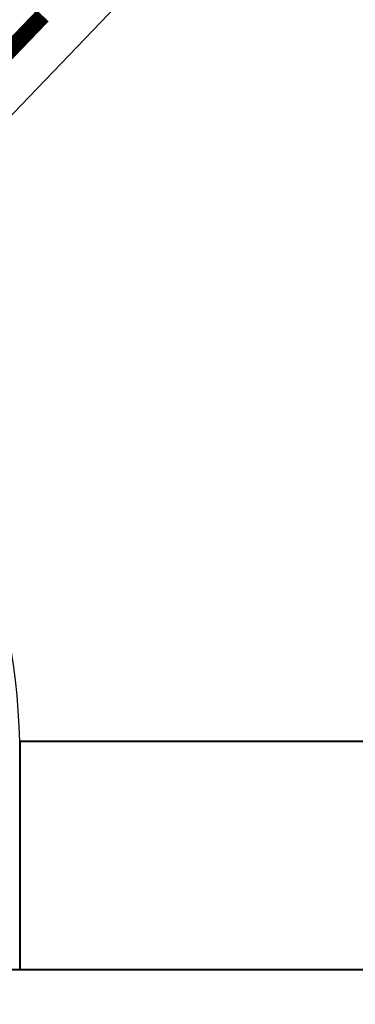
# Model space of a CAD drawing. Units: inches. Extents: x 459864 to 460310, y 324185 to 324787.
# Tile 64 of 112: x 460088 to 460101, y 324282 to 324321. Entities that reach past the tile are written whole.
import ezdxf

# ---------------------------------------------------------------- set-up
doc = ezdxf.new("R2010")
doc.units = ezdxf.units.IN
for name, color, linetype, lineweight in [('A-ANNO-DIMS', 2, 'Continuous', 18), ('A-DOOR', 3, 'Continuous', 25), ('A-WALL', 7, 'Continuous', 40), ('L-SITE-PATT', 252, 'Continuous', 13)]:
    doc.layers.add(name, color=color, linetype=linetype, lineweight=lineweight)
doc.styles.get("Standard").update_dxf_attribs({"font": 'arial.ttf'})
doc.dimstyles.new('ISO-25', dxfattribs={"dimtxt": 6, "dimasz": 2.5, "dimexe": 1.25, "dimexo": 0.625, "dimtad": 1, "dimdec": 1, "dimlunit": 3, "dimtxsty": 'Standard', "dimcen": 2.5, "dimadec": 0, "dimazin": 0, "dimtfac": 1, "dimtdec": 1, "dimtmove": 0, "dimatfit": 3, "dimfxl": 1, "dimarcsym": 0})

# ---------------------------------------------------------------- blocks, each defined once
blk = doc.blocks.new('*D73')
at = {"layer": 'A-ANNO-DIMS', "color": 0, "lineweight": -2, "transparency": 16777216}
for p, q in [((460109.617, 324339.904), (460082.316, 324311.465)), ((460063.615, 324291.983), (460080.585, 324309.661))]:
    blk.add_line(p, q, dxfattribs=at)
at = {"layer": 'A-ANNO-DIMS', "color": 0, "transparency": 16777216}
blk.add_solid([(460082.016, 324311.753), (460082.617, 324311.176), (460080.585, 324309.661)], dxfattribs=at)
at = {"layer": 'Defpoints', "color": 0, "transparency": 16777216}
for p in [(460080.585, 324309.661), (460063.615, 324291.983)]:
    blk.add_point(p, dxfattribs=at)
at = {"layer": 'A-ANNO-DIMS', "color": 0, "transparency": 16777216, "insert": (460094.144, 324329.167), "char_height": 6, "attachment_point": 5, "rotation": 46.1701}
blk.add_mtext('R2\'-0 1/2"', dxfattribs=at)

msp = doc.modelspace()

# ---------------------------------------------------------------- hatches: boundary and pattern name
at = {"layer": 'L-SITE-PATT'}
h = msp.add_hatch(dxfattribs=at)
h.set_pattern_fill('DOTS', color=256)
h.paths.add_polyline_path([(460269.804, 324283.483), (460247.115, 324283.483), (460121.929, 324283.483), (460121.929, 324252.473), (460117.429, 324252.473), (460110.124, 324252.473), (460110.124, 324243.287), (460080.83, 324243.287), (460080.83, 324252.473), (460061.115, 324252.473), (460061.115, 324251.882), (460077.909, 324251.882), (460077.909, 324199.483), (460080.83, 324199.483), (460080.83, 324207.553), (460110.124, 324207.553), (460110.124, 324199.483), (460110.813, 324199.483), (460262.115, 324199.483), (460269.804, 324199.483)], flags=17)
edge = h.paths.add_edge_path(flags=0)
edge.add_ellipse((460222.59, 324263.813), major_axis=(-8.485, 8.485), ratio=1, start_angle=405, end_angle=495, ccw=False)
edge.add_line((460214.821, 324254.66), (460214.832, 324254.666))
edge.add_ellipse((460222.59, 324263.813), major_axis=(-8.485, 8.485), ratio=1, start_angle=405, end_angle=495, ccw=False)
edge.add_line((460210.759, 324261.781), (460210.768, 324261.787))
edge.add_ellipse((460222.59, 324263.813), major_axis=(-8.485, 8.485), ratio=1, start_angle=405, end_angle=495, ccw=False)
edge.add_ellipse((460222.59, 324263.813), major_axis=(-8.485, 8.485), ratio=1, start_angle=392.754, end_angle=405, ccw=False)
edge.add_ellipse((460222.59, 324263.813), major_axis=(-8.485, 8.485), ratio=1, start_angle=380.9347, end_angle=392.754, ccw=False)
edge.add_line((460211.337, 324267.985), (460211.34, 324267.985))
edge.add_ellipse((460222.59, 324263.813), major_axis=(-8.485, 8.485), ratio=1, start_angle=380.9347, end_angle=392.754, ccw=False)
edge.add_ellipse((460222.59, 324263.813), major_axis=(-8.485, 8.485), ratio=1, start_angle=347.9015, end_angle=380.9347, ccw=False)
edge.add_ellipse((460222.59, 324263.813), major_axis=(-8.485, 8.485), ratio=1, start_angle=327.0619, end_angle=347.9015, ccw=False)
edge.add_ellipse((460222.59, 324263.813), major_axis=(-8.485, 8.485), ratio=1, start_angle=278.3246, end_angle=327.0619, ccw=False)
edge.add_line((460225.158, 324275.536), (460225.158, 324275.535))
edge.add_ellipse((460222.59, 324263.813), major_axis=(-8.485, 8.485), ratio=1, start_angle=278.3246, end_angle=327.0619, ccw=False)
edge.add_ellipse((460222.59, 324263.813), major_axis=(-8.485, 8.485), ratio=1, start_angle=260.6436, end_angle=278.3246, ccw=False)
edge.add_ellipse((460222.59, 324263.813), major_axis=(-8.485, 8.485), ratio=1, start_angle=225, end_angle=260.6436, ccw=False)
edge.add_line((460234.509, 324265.243), (460234.501, 324265.239))
edge.add_ellipse((460222.59, 324263.813), major_axis=(-8.485, 8.485), ratio=1, start_angle=225, end_angle=260.6436, ccw=False)
edge.add_ellipse((460222.59, 324263.813), major_axis=(-8.485, 8.485), ratio=1, start_angle=495, end_angle=585, ccw=False)
edge.add_line((460234.437, 324261.861), (460234.424, 324261.858))
edge.add_ellipse((460222.59, 324263.813), major_axis=(-8.485, 8.485), ratio=1, start_angle=495, end_angle=585, ccw=False)
edge.add_line((460227.95, 324253.067), (460227.946, 324253.083))
edge.add_ellipse((460222.59, 324263.813), major_axis=(-8.485, 8.485), ratio=1, start_angle=495, end_angle=585, ccw=False)
edge.add_line((460226.223, 324252.369), (460226.211, 324252.38))
edge.add_ellipse((460222.59, 324263.813), major_axis=(-8.485, 8.485), ratio=1, start_angle=495, end_angle=585, ccw=False)
h.paths.add_polyline_path([(460219.651, 324254.347), (460218.461, 324253.545), (460218.275, 324254.789), (460219.642, 324256.542), (460219.625, 324260.848), (460216.11, 324257.333), (460214.35, 324256.978), (460215.416, 324259.356), (460212.524, 324258.496), (460213.137, 324259.93), (460218.507, 324263.813), (460222.59, 324263.813), (460222.59, 324267.807), (460218.176, 324272.212), (460219.026, 324274.639), (460222.59, 324272.811), (460222.59, 324275.423), (460223.057, 324274.825), (460222.675, 324273.492), (460225.912, 324267.135), (460219.625, 324260.848)], flags=0)
edge = h.paths.add_edge_path(flags=0)
edge.add_ellipse((460194.576, 324264.046), major_axis=(-8.485, 8.485), ratio=1, start_angle=495, end_angle=585, ccw=False)
edge.add_line((460199.936, 324253.3), (460199.932, 324253.316))
edge.add_ellipse((460194.576, 324264.046), major_axis=(-8.485, 8.485), ratio=1, start_angle=495, end_angle=585, ccw=False)
edge.add_line((460198.208, 324252.603), (460198.196, 324252.613))
edge.add_ellipse((460194.576, 324264.046), major_axis=(-8.485, 8.485), ratio=1, start_angle=495, end_angle=585, ccw=False)
edge.add_ellipse((460194.576, 324264.046), major_axis=(-8.485, 8.485), ratio=1, start_angle=405, end_angle=495, ccw=False)
edge.add_line((460186.806, 324254.893), (460186.817, 324254.899))
edge.add_ellipse((460194.576, 324264.046), major_axis=(-8.485, 8.485), ratio=1, start_angle=405, end_angle=495, ccw=False)
edge.add_line((460182.744, 324262.014), (460182.753, 324262.02))
edge.add_ellipse((460194.576, 324264.046), major_axis=(-8.485, 8.485), ratio=1, start_angle=405, end_angle=495, ccw=False)
edge.add_ellipse((460194.576, 324264.046), major_axis=(-8.485, 8.485), ratio=1, start_angle=392.754, end_angle=405, ccw=False)
edge.add_ellipse((460194.576, 324264.046), major_axis=(-8.485, 8.485), ratio=1, start_angle=380.9347, end_angle=392.754, ccw=False)
edge.add_line((460183.323, 324268.218), (460183.326, 324268.218))
edge.add_ellipse((460194.576, 324264.046), major_axis=(-8.485, 8.485), ratio=1, start_angle=380.9347, end_angle=392.754, ccw=False)
edge.add_ellipse((460194.576, 324264.046), major_axis=(-8.485, 8.485), ratio=1, start_angle=347.9015, end_angle=380.9347, ccw=False)
edge.add_ellipse((460194.576, 324264.046), major_axis=(-8.485, 8.485), ratio=1, start_angle=327.0619, end_angle=347.9015, ccw=False)
edge.add_ellipse((460194.576, 324264.046), major_axis=(-8.485, 8.485), ratio=1, start_angle=278.3246, end_angle=327.0619, ccw=False)
edge.add_line((460197.144, 324275.769), (460197.143, 324275.768))
edge.add_ellipse((460194.576, 324264.046), major_axis=(-8.485, 8.485), ratio=1, start_angle=278.3246, end_angle=327.0619, ccw=False)
edge.add_ellipse((460194.576, 324264.046), major_axis=(-8.485, 8.485), ratio=1, start_angle=260.6436, end_angle=278.3246, ccw=False)
edge.add_ellipse((460194.576, 324264.046), major_axis=(-8.485, 8.485), ratio=1, start_angle=225, end_angle=260.6436, ccw=False)
edge.add_line((460206.494, 324265.476), (460206.487, 324265.473))
edge.add_ellipse((460194.576, 324264.046), major_axis=(-8.485, 8.485), ratio=1, start_angle=225, end_angle=260.6436, ccw=False)
edge.add_ellipse((460194.576, 324264.046), major_axis=(-8.485, 8.485), ratio=1, start_angle=495, end_angle=585, ccw=False)
edge.add_line((460206.422, 324262.094), (460206.409, 324262.091))
h.paths.add_polyline_path([(460191.61, 324261.081), (460191.637, 324254.58), (460190.447, 324253.778), (460190.261, 324255.023), (460191.628, 324256.775), (460191.61, 324261.081), (460188.096, 324257.566), (460186.335, 324257.211), (460187.402, 324259.589), (460184.509, 324258.729), (460185.123, 324260.163), (460190.493, 324264.046), (460194.576, 324264.046), (460194.576, 324268.04), (460190.161, 324272.446), (460191.011, 324274.872), (460194.576, 324273.044), (460194.576, 324275.657), (460195.043, 324275.058), (460194.661, 324273.725), (460197.897, 324267.368)], flags=0)
edge = h.paths.add_edge_path(flags=0)
edge.add_ellipse((460252.912, 324263.578), major_axis=(-8.485, 8.485), ratio=1, start_angle=405, end_angle=495, ccw=False)
edge.add_line((460241.081, 324261.545), (460241.089, 324261.551))
edge.add_ellipse((460252.912, 324263.578), major_axis=(-8.485, 8.485), ratio=1, start_angle=405, end_angle=495, ccw=False)
edge.add_ellipse((460252.912, 324263.578), major_axis=(-8.485, 8.485), ratio=1, start_angle=392.754, end_angle=405, ccw=False)
edge.add_ellipse((460252.912, 324263.578), major_axis=(-8.485, 8.485), ratio=1, start_angle=380.9347, end_angle=392.754, ccw=False)
edge.add_line((460241.659, 324267.749), (460241.662, 324267.749))
edge.add_ellipse((460252.912, 324263.578), major_axis=(-8.485, 8.485), ratio=1, start_angle=380.9347, end_angle=392.754, ccw=False)
edge.add_ellipse((460252.912, 324263.578), major_axis=(-8.485, 8.485), ratio=1, start_angle=347.9015, end_angle=380.9347, ccw=False)
edge.add_ellipse((460252.912, 324263.578), major_axis=(-8.485, 8.485), ratio=1, start_angle=327.0619, end_angle=347.9015, ccw=False)
edge.add_ellipse((460252.912, 324263.578), major_axis=(-8.485, 8.485), ratio=1, start_angle=278.3246, end_angle=327.0619, ccw=False)
edge.add_line((460255.48, 324275.3), (460255.479, 324275.299))
edge.add_ellipse((460252.912, 324263.578), major_axis=(-8.485, 8.485), ratio=1, start_angle=278.3246, end_angle=327.0619, ccw=False)
edge.add_ellipse((460252.912, 324263.578), major_axis=(-8.485, 8.485), ratio=1, start_angle=260.6436, end_angle=278.3246, ccw=False)
edge.add_ellipse((460252.912, 324263.578), major_axis=(-8.485, 8.485), ratio=1, start_angle=225, end_angle=260.6436, ccw=False)
edge.add_line((460264.83, 324265.007), (460264.823, 324265.004))
edge.add_ellipse((460252.912, 324263.578), major_axis=(-8.485, 8.485), ratio=1, start_angle=225, end_angle=260.6436, ccw=False)
edge.add_ellipse((460252.912, 324263.578), major_axis=(-8.485, 8.485), ratio=1, start_angle=495, end_angle=585, ccw=False)
edge.add_line((460264.758, 324261.626), (460264.745, 324261.622))
edge.add_ellipse((460252.912, 324263.578), major_axis=(-8.485, 8.485), ratio=1, start_angle=495, end_angle=585, ccw=False)
edge.add_line((460258.272, 324252.832), (460258.268, 324252.848))
edge.add_ellipse((460252.912, 324263.578), major_axis=(-8.485, 8.485), ratio=1, start_angle=495, end_angle=585, ccw=False)
edge.add_line((460256.545, 324252.134), (460256.533, 324252.144))
edge.add_ellipse((460252.912, 324263.578), major_axis=(-8.485, 8.485), ratio=1, start_angle=495, end_angle=585, ccw=False)
edge.add_ellipse((460252.912, 324263.578), major_axis=(-8.485, 8.485), ratio=1, start_angle=405, end_angle=495, ccw=False)
edge.add_line((460245.143, 324254.424), (460245.153, 324254.43))
h.paths.add_polyline_path([(460244.672, 324256.742), (460245.738, 324259.12), (460242.846, 324258.26), (460243.459, 324259.694), (460248.829, 324263.578), (460252.912, 324263.578), (460252.912, 324267.571), (460248.497, 324271.977), (460249.348, 324274.403), (460252.912, 324272.576), (460252.912, 324275.188), (460253.379, 324274.589), (460252.997, 324273.257), (460256.233, 324266.899), (460249.946, 324260.612), (460249.973, 324254.111), (460248.783, 324253.309), (460248.597, 324254.554), (460249.964, 324256.306), (460249.946, 324260.612), (460246.432, 324257.097)], flags=0)
edge = h.paths.add_edge_path(flags=0)
edge.add_ellipse((460167.439, 324262.833), major_axis=(-8.485, 8.485), ratio=1, start_angle=495, end_angle=585, ccw=False)
edge.add_line((460172.799, 324252.087), (460172.795, 324252.103))
edge.add_ellipse((460167.439, 324262.833), major_axis=(-8.485, 8.485), ratio=1, start_angle=495, end_angle=585, ccw=False)
edge.add_line((460171.071, 324251.389), (460171.059, 324251.399))
edge.add_ellipse((460167.439, 324262.833), major_axis=(-8.485, 8.485), ratio=1, start_angle=495, end_angle=585, ccw=False)
edge.add_ellipse((460167.439, 324262.833), major_axis=(-8.485, 8.485), ratio=1, start_angle=405, end_angle=495, ccw=False)
edge.add_line((460159.669, 324253.679), (460159.68, 324253.685))
edge.add_ellipse((460167.439, 324262.833), major_axis=(-8.485, 8.485), ratio=1, start_angle=405, end_angle=495, ccw=False)
edge.add_line((460155.607, 324260.8), (460155.616, 324260.806))
edge.add_ellipse((460167.439, 324262.833), major_axis=(-8.485, 8.485), ratio=1, start_angle=405, end_angle=495, ccw=False)
edge.add_ellipse((460167.439, 324262.833), major_axis=(-8.485, 8.485), ratio=1, start_angle=392.754, end_angle=405, ccw=False)
edge.add_ellipse((460167.439, 324262.833), major_axis=(-8.485, 8.485), ratio=1, start_angle=380.9347, end_angle=392.754, ccw=False)
edge.add_line((460156.185, 324267.005), (460156.189, 324267.005))
edge.add_ellipse((460167.439, 324262.833), major_axis=(-8.485, 8.485), ratio=1, start_angle=380.9347, end_angle=392.754, ccw=False)
edge.add_ellipse((460167.439, 324262.833), major_axis=(-8.485, 8.485), ratio=1, start_angle=347.9015, end_angle=380.9347, ccw=False)
edge.add_ellipse((460167.439, 324262.833), major_axis=(-8.485, 8.485), ratio=1, start_angle=327.0619, end_angle=347.9015, ccw=False)
edge.add_ellipse((460167.439, 324262.833), major_axis=(-8.485, 8.485), ratio=1, start_angle=278.3246, end_angle=327.0619, ccw=False)
edge.add_line((460170.007, 324274.556), (460170.006, 324274.554))
edge.add_ellipse((460167.439, 324262.833), major_axis=(-8.485, 8.485), ratio=1, start_angle=278.3246, end_angle=327.0619, ccw=False)
edge.add_ellipse((460167.439, 324262.833), major_axis=(-8.485, 8.485), ratio=1, start_angle=260.6436, end_angle=278.3246, ccw=False)
edge.add_ellipse((460167.439, 324262.833), major_axis=(-8.485, 8.485), ratio=1, start_angle=225, end_angle=260.6436, ccw=False)
edge.add_line((460179.357, 324264.262), (460179.35, 324264.259))
edge.add_ellipse((460167.439, 324262.833), major_axis=(-8.485, 8.485), ratio=1, start_angle=225, end_angle=260.6436, ccw=False)
edge.add_ellipse((460167.439, 324262.833), major_axis=(-8.485, 8.485), ratio=1, start_angle=495, end_angle=585, ccw=False)
edge.add_line((460179.285, 324260.881), (460179.272, 324260.877))
h.paths.add_polyline_path([(460164.473, 324259.867), (460164.5, 324253.366), (460163.31, 324252.565), (460163.124, 324253.809), (460164.491, 324255.561), (460164.473, 324259.867), (460160.958, 324256.353), (460159.198, 324255.998), (460160.265, 324258.375), (460157.372, 324257.515), (460157.986, 324258.949), (460163.356, 324262.833), (460167.439, 324262.833), (460167.439, 324266.826), (460163.024, 324271.232), (460163.874, 324273.659), (460167.439, 324271.831), (460167.439, 324274.443), (460167.905, 324273.844), (460167.524, 324272.512), (460170.76, 324266.154)], flags=0)
edge = h.paths.add_edge_path(flags=0)
edge.add_ellipse((460140.758, 324262.37), major_axis=(-8.485, 8.485), ratio=1, start_angle=495, end_angle=585, ccw=False)
edge.add_line((460146.118, 324251.624), (460146.114, 324251.639))
edge.add_ellipse((460140.758, 324262.37), major_axis=(-8.485, 8.485), ratio=1, start_angle=495, end_angle=585, ccw=False)
edge.add_line((460144.391, 324250.926), (460144.379, 324250.936))
edge.add_ellipse((460140.758, 324262.37), major_axis=(-8.485, 8.485), ratio=1, start_angle=495, end_angle=585, ccw=False)
edge.add_ellipse((460140.758, 324262.37), major_axis=(-8.485, 8.485), ratio=1, start_angle=405, end_angle=495, ccw=False)
edge.add_line((460132.989, 324253.216), (460132.999, 324253.222))
edge.add_ellipse((460140.758, 324262.37), major_axis=(-8.485, 8.485), ratio=1, start_angle=405, end_angle=495, ccw=False)
edge.add_line((460128.927, 324260.337), (460128.935, 324260.343))
edge.add_ellipse((460140.758, 324262.37), major_axis=(-8.485, 8.485), ratio=1, start_angle=405, end_angle=495, ccw=False)
edge.add_ellipse((460140.758, 324262.37), major_axis=(-8.485, 8.485), ratio=1, start_angle=392.754, end_angle=405, ccw=False)
edge.add_ellipse((460140.758, 324262.37), major_axis=(-8.485, 8.485), ratio=1, start_angle=380.9347, end_angle=392.754, ccw=False)
edge.add_line((460129.505, 324266.541), (460129.508, 324266.541))
edge.add_ellipse((460140.758, 324262.37), major_axis=(-8.485, 8.485), ratio=1, start_angle=380.9347, end_angle=392.754, ccw=False)
edge.add_ellipse((460140.758, 324262.37), major_axis=(-8.485, 8.485), ratio=1, start_angle=347.9015, end_angle=380.9347, ccw=False)
edge.add_ellipse((460140.758, 324262.37), major_axis=(-8.485, 8.485), ratio=1, start_angle=327.0619, end_angle=347.9015, ccw=False)
edge.add_ellipse((460140.758, 324262.37), major_axis=(-8.485, 8.485), ratio=1, start_angle=278.3246, end_angle=327.0619, ccw=False)
edge.add_line((460143.326, 324274.092), (460143.325, 324274.091))
edge.add_ellipse((460140.758, 324262.37), major_axis=(-8.485, 8.485), ratio=1, start_angle=278.3246, end_angle=327.0619, ccw=False)
edge.add_ellipse((460140.758, 324262.37), major_axis=(-8.485, 8.485), ratio=1, start_angle=260.6436, end_angle=278.3246, ccw=False)
edge.add_ellipse((460140.758, 324262.37), major_axis=(-8.485, 8.485), ratio=1, start_angle=225, end_angle=260.6436, ccw=False)
edge.add_line((460152.677, 324263.799), (460152.669, 324263.796))
edge.add_ellipse((460140.758, 324262.37), major_axis=(-8.485, 8.485), ratio=1, start_angle=225, end_angle=260.6436, ccw=False)
edge.add_ellipse((460140.758, 324262.37), major_axis=(-8.485, 8.485), ratio=1, start_angle=495, end_angle=585, ccw=False)
edge.add_line((460152.604, 324260.418), (460152.592, 324260.414))
h.paths.add_polyline_path([(460137.792, 324259.404), (460137.819, 324252.903), (460136.629, 324252.101), (460136.443, 324253.346), (460137.81, 324255.098), (460137.792, 324259.404), (460134.278, 324255.889), (460132.518, 324255.534), (460133.584, 324257.912), (460130.692, 324257.052), (460131.305, 324258.486), (460136.675, 324262.37), (460140.758, 324262.37), (460140.758, 324266.363), (460136.343, 324270.769), (460137.194, 324273.195), (460140.758, 324271.367), (460140.758, 324273.98), (460141.225, 324273.381), (460140.843, 324272.049), (460144.079, 324265.691)], flags=0)
h.paths.add_polyline_path([(460110.124, 324227.414), (460080.83, 324227.414), (460080.83, 324235.484), (460110.124, 324235.484)], flags=16)
h.paths.add_polyline_path([(460110.124, 324220.797), (460110.124, 324212.727), (460080.83, 324212.727), (460080.83, 324220.797)], flags=16)
h.paths.add_polyline_path([(460269.804, 324283.483), (460247.115, 324283.483), (460121.929, 324283.483), (460121.929, 324252.473), (460117.429, 324252.473), (460110.124, 324252.473), (460110.124, 324243.287), (460080.83, 324243.287), (460080.83, 324252.473), (460061.115, 324252.473), (460061.115, 324251.882), (460077.909, 324251.882), (460077.909, 324199.483), (460080.83, 324199.483), (460080.83, 324207.553), (460110.124, 324207.553), (460110.124, 324199.483), (460262.115, 324199.483), (460269.804, 324199.483)], flags=17)
h.paths.add_polyline_path([(460219.651, 324254.347), (460218.461, 324253.545), (460218.275, 324254.789), (460219.642, 324256.542), (460219.625, 324260.848), (460216.11, 324257.333), (460214.35, 324256.978), (460215.416, 324259.356), (460212.524, 324258.496), (460213.137, 324259.93), (460218.507, 324263.813), (460222.59, 324263.813), (460220.18, 324266.223), (460215.461, 324265.308), (460211.835, 324266.137), (460216.247, 324267.985), (460218.418, 324267.985), (460222.59, 324263.813), (460222.59, 324267.807), (460218.176, 324272.212), (460219.026, 324274.639), (460222.59, 324272.811), (460222.59, 324275.423), (460223.057, 324274.825), (460222.675, 324273.492), (460225.912, 324267.135), (460222.59, 324263.813), (460231.383, 324263.813), (460228.485, 324262.488), (460224.425, 324261.978), (460228.68, 324257.724), (460228.966, 324254.791), (460227.142, 324256.537), (460227.542, 324254.819), (460227.333, 324253.614), (460222.59, 324259.985), (460222.59, 324255.497), (460221.377, 324256.541), (460220.576, 324261.799), (460219.625, 324260.848)], flags=0)
h.paths.add_polyline_path([(460199.127, 324256.77), (460199.528, 324255.052), (460199.319, 324253.848), (460194.576, 324260.218), (460194.576, 324255.73), (460193.363, 324256.774), (460192.561, 324262.032), (460191.61, 324261.081), (460191.637, 324254.58), (460190.447, 324253.778), (460190.261, 324255.023), (460191.628, 324256.775), (460191.61, 324261.081), (460188.096, 324257.566), (460186.335, 324257.211), (460187.402, 324259.589), (460184.509, 324258.729), (460185.123, 324260.163), (460190.493, 324264.046), (460194.576, 324264.046), (460192.166, 324266.456), (460187.446, 324265.541), (460183.82, 324266.37), (460188.232, 324268.218), (460190.404, 324268.218), (460194.576, 324264.046), (460194.576, 324268.04), (460190.161, 324272.446), (460191.011, 324274.872), (460194.576, 324273.044), (460194.576, 324275.657), (460195.043, 324275.058), (460194.661, 324273.725), (460197.897, 324267.368), (460194.576, 324264.046), (460203.368, 324264.046), (460200.47, 324262.721), (460196.411, 324262.212), (460200.665, 324257.957), (460200.951, 324255.024)], flags=0)
h.paths.add_polyline_path([(460244.672, 324256.742), (460245.738, 324259.12), (460242.846, 324258.26), (460243.459, 324259.694), (460248.829, 324263.578), (460252.912, 324263.578), (460250.502, 324265.987), (460245.783, 324265.072), (460242.156, 324265.901), (460246.568, 324267.749), (460248.74, 324267.749), (460252.912, 324263.578), (460252.912, 324267.571), (460248.497, 324271.977), (460249.348, 324274.403), (460252.912, 324272.576), (460252.912, 324275.188), (460253.379, 324274.589), (460252.997, 324273.257), (460256.233, 324266.899), (460252.912, 324263.578), (460261.705, 324263.578), (460258.806, 324262.252), (460254.747, 324261.743), (460259.002, 324257.488), (460259.288, 324254.555), (460257.463, 324256.301), (460257.864, 324254.583), (460257.655, 324253.379), (460252.912, 324259.749), (460252.912, 324255.261), (460251.699, 324256.305), (460250.897, 324261.563), (460249.946, 324260.612), (460249.973, 324254.111), (460248.783, 324253.309), (460248.597, 324254.554), (460249.964, 324256.306), (460249.946, 324260.612), (460246.432, 324257.097)], flags=0)
h.paths.add_polyline_path([(460173.528, 324256.743), (460173.814, 324253.811), (460171.99, 324255.556), (460172.39, 324253.838), (460172.182, 324252.634), (460167.439, 324259.004), (460167.439, 324254.516), (460166.226, 324255.56), (460165.424, 324260.818), (460164.473, 324259.867), (460164.5, 324253.366), (460163.31, 324252.565), (460163.124, 324253.809), (460164.491, 324255.561), (460164.473, 324259.867), (460160.958, 324256.353), (460159.198, 324255.998), (460160.265, 324258.375), (460157.372, 324257.515), (460157.986, 324258.949), (460163.356, 324262.833), (460167.439, 324262.833), (460165.029, 324265.243), (460160.309, 324264.327), (460156.683, 324265.156), (460161.095, 324267.005), (460163.267, 324267.005), (460167.439, 324262.833), (460167.439, 324266.826), (460163.024, 324271.232), (460163.874, 324273.659), (460167.439, 324271.831), (460167.439, 324274.443), (460167.905, 324273.844), (460167.524, 324272.512), (460170.76, 324266.154), (460167.439, 324262.833), (460176.231, 324262.833), (460173.333, 324261.507), (460169.274, 324260.998)], flags=0)
h.paths.add_polyline_path([(460146.848, 324256.28), (460147.134, 324253.347), (460145.31, 324255.093), (460145.71, 324253.375), (460145.501, 324252.171), (460140.758, 324258.541), (460140.758, 324254.053), (460139.545, 324255.097), (460138.744, 324260.355), (460137.792, 324259.404), (460137.819, 324252.903), (460136.629, 324252.101), (460136.443, 324253.346), (460137.81, 324255.098), (460137.792, 324259.404), (460134.278, 324255.889), (460132.518, 324255.534), (460133.584, 324257.912), (460130.692, 324257.052), (460131.305, 324258.486), (460136.675, 324262.37), (460140.758, 324262.37), (460138.348, 324264.779), (460133.629, 324263.864), (460130.002, 324264.693), (460134.414, 324266.541), (460136.586, 324266.541), (460140.758, 324262.37), (460140.758, 324266.363), (460136.343, 324270.769), (460137.194, 324273.195), (460140.758, 324271.367), (460140.758, 324273.98), (460141.225, 324273.381), (460140.843, 324272.049), (460144.079, 324265.691), (460140.758, 324262.37), (460149.551, 324262.37), (460146.653, 324261.044), (460142.593, 324260.535)], flags=0)
edge = h.paths.add_edge_path()
edge.add_line((460269.804, 324272.549), (460260.881, 324272.549))
edge.add_ellipse((460252.912, 324263.578), major_axis=(-8.485, 8.485), ratio=1, start_angle=260.6436, end_angle=273.3846, ccw=False)
edge.add_line((460262.283, 324271.092), (460262.261, 324271.091))
edge.add_ellipse((460252.912, 324263.578), major_axis=(-8.485, 8.485), ratio=1, start_angle=260.6436, end_angle=273.3846, ccw=False)
edge.add_ellipse((460252.912, 324263.578), major_axis=(-8.485, 8.485), ratio=1, start_angle=225, end_angle=260.6436, ccw=False)
edge.add_line((460263.609, 324269.063), (460263.572, 324269.058))
edge.add_ellipse((460252.912, 324263.578), major_axis=(-8.485, 8.485), ratio=1, start_angle=225, end_angle=260.6436, ccw=False)
edge.add_line((460264.615, 324266.306), (460264.585, 324266.305))
edge.add_ellipse((460252.912, 324263.578), major_axis=(-8.485, 8.485), ratio=1, start_angle=225, end_angle=260.6436, ccw=False)
edge.add_line((460264.83, 324265.007), (460264.823, 324265.004))
edge.add_ellipse((460252.912, 324263.578), major_axis=(-8.485, 8.485), ratio=1, start_angle=225, end_angle=260.6436, ccw=False)
edge.add_ellipse((460252.912, 324263.578), major_axis=(-8.485, 8.485), ratio=1, start_angle=495, end_angle=585, ccw=False)
edge.add_line((460264.758, 324261.626), (460264.745, 324261.622))
edge.add_ellipse((460252.912, 324263.578), major_axis=(-8.485, 8.485), ratio=1, start_angle=495, end_angle=585, ccw=False)
edge.add_line((460263.442, 324257.739), (460263.389, 324257.779))
edge.add_ellipse((460252.912, 324263.578), major_axis=(-8.485, 8.485), ratio=1, start_angle=495, end_angle=585, ccw=False)
edge.add_line((460258.128, 324252.744), (460258.102, 324252.779))
edge.add_ellipse((460252.912, 324263.578), major_axis=(-8.485, 8.485), ratio=1, start_angle=495, end_angle=585, ccw=False)
edge.add_line((460256.545, 324252.134), (460256.533, 324252.144))
edge.add_ellipse((460252.912, 324263.578), major_axis=(-8.485, 8.485), ratio=1, start_angle=495, end_angle=585, ccw=False)
edge.add_ellipse((460252.912, 324263.578), major_axis=(-8.485, 8.485), ratio=1, start_angle=405, end_angle=495, ccw=False)
edge.add_line((460250.594, 324251.78), (460250.605, 324251.82))
edge.add_ellipse((460252.912, 324263.578), major_axis=(-8.485, 8.485), ratio=1, start_angle=405, end_angle=495, ccw=False)
edge.add_line((460245.143, 324254.424), (460245.153, 324254.43))
edge.add_ellipse((460252.912, 324263.578), major_axis=(-8.485, 8.485), ratio=1, start_angle=405, end_angle=495, ccw=False)
edge.add_line((460243.525, 324256.059), (460243.56, 324256.091))
edge.add_ellipse((460252.912, 324263.578), major_axis=(-8.485, 8.485), ratio=1, start_angle=405, end_angle=495, ccw=False)
edge.add_line((460241.44, 324259.893), (460241.522, 324259.896))
edge.add_ellipse((460252.912, 324263.578), major_axis=(-8.485, 8.485), ratio=1, start_angle=405, end_angle=495, ccw=False)
edge.add_line((460241.081, 324261.545), (460241.089, 324261.551))
edge.add_ellipse((460252.912, 324263.578), major_axis=(-8.485, 8.485), ratio=1, start_angle=405, end_angle=495, ccw=False)
edge.add_ellipse((460252.912, 324263.578), major_axis=(-8.485, 8.485), ratio=1, start_angle=392.754, end_angle=405, ccw=False)
edge.add_line((460241.05, 324265.438), (460241.063, 324265.443))
edge.add_ellipse((460252.912, 324263.578), major_axis=(-8.485, 8.485), ratio=1, start_angle=392.754, end_angle=405, ccw=False)
edge.add_ellipse((460252.912, 324263.578), major_axis=(-8.485, 8.485), ratio=1, start_angle=380.9347, end_angle=392.754, ccw=False)
edge.add_line((460241.452, 324267.176), (460241.469, 324267.171))
edge.add_ellipse((460252.912, 324263.578), major_axis=(-8.485, 8.485), ratio=1, start_angle=380.9347, end_angle=392.754, ccw=False)
edge.add_line((460241.659, 324267.749), (460241.662, 324267.749))
edge.add_ellipse((460252.912, 324263.578), major_axis=(-8.485, 8.485), ratio=1, start_angle=380.9347, end_angle=392.754, ccw=False)
edge.add_ellipse((460252.912, 324263.578), major_axis=(-8.485, 8.485), ratio=1, start_angle=356.6154, end_angle=380.9347, ccw=False)
edge.add_line((460244.88, 324272.488), (460244.713, 324272.549))
edge.add_line((460244.713, 324272.549), (460230.817, 324272.549))
edge.add_ellipse((460222.59, 324263.813), major_axis=(-8.485, 8.485), ratio=1, start_angle=260.6436, end_angle=271.7178, ccw=False)
edge.add_ellipse((460222.59, 324263.813), major_axis=(-8.485, 8.485), ratio=1, start_angle=225, end_angle=260.6436, ccw=False)
edge.add_line((460233.287, 324269.299), (460233.25, 324269.294))
edge.add_ellipse((460222.59, 324263.813), major_axis=(-8.485, 8.485), ratio=1, start_angle=225, end_angle=260.6436, ccw=False)
edge.add_line((460234.294, 324266.541), (460234.264, 324266.541))
edge.add_ellipse((460222.59, 324263.813), major_axis=(-8.485, 8.485), ratio=1, start_angle=225, end_angle=260.6436, ccw=False)
edge.add_line((460234.509, 324265.243), (460234.501, 324265.239))
edge.add_ellipse((460222.59, 324263.813), major_axis=(-8.485, 8.485), ratio=1, start_angle=225, end_angle=260.6436, ccw=False)
edge.add_ellipse((460222.59, 324263.813), major_axis=(-8.485, 8.485), ratio=1, start_angle=495, end_angle=585, ccw=False)
edge.add_line((460234.437, 324261.861), (460234.424, 324261.858))
edge.add_ellipse((460222.59, 324263.813), major_axis=(-8.485, 8.485), ratio=1, start_angle=495, end_angle=585, ccw=False)
edge.add_line((460233.121, 324257.975), (460233.068, 324258.015))
edge.add_ellipse((460222.59, 324263.813), major_axis=(-8.485, 8.485), ratio=1, start_angle=495, end_angle=585, ccw=False)
edge.add_line((460227.806, 324252.979), (460227.78, 324253.014))
edge.add_ellipse((460222.59, 324263.813), major_axis=(-8.485, 8.485), ratio=1, start_angle=495, end_angle=585, ccw=False)
edge.add_line((460226.223, 324252.369), (460226.211, 324252.38))
edge.add_ellipse((460222.59, 324263.813), major_axis=(-8.485, 8.485), ratio=1, start_angle=495, end_angle=585, ccw=False)
edge.add_ellipse((460222.59, 324263.813), major_axis=(-8.485, 8.485), ratio=1, start_angle=405, end_angle=495, ccw=False)
edge.add_line((460220.272, 324252.016), (460220.283, 324252.055))
edge.add_ellipse((460222.59, 324263.813), major_axis=(-8.485, 8.485), ratio=1, start_angle=405, end_angle=495, ccw=False)
edge.add_line((460214.821, 324254.66), (460214.832, 324254.666))
edge.add_ellipse((460222.59, 324263.813), major_axis=(-8.485, 8.485), ratio=1, start_angle=405, end_angle=495, ccw=False)
edge.add_line((460213.203, 324256.295), (460213.239, 324256.327))
edge.add_ellipse((460222.59, 324263.813), major_axis=(-8.485, 8.485), ratio=1, start_angle=405, end_angle=495, ccw=False)
edge.add_line((460211.118, 324260.128), (460211.201, 324260.131))
edge.add_ellipse((460222.59, 324263.813), major_axis=(-8.485, 8.485), ratio=1, start_angle=405, end_angle=495, ccw=False)
edge.add_line((460210.759, 324261.781), (460210.768, 324261.787))
edge.add_ellipse((460222.59, 324263.813), major_axis=(-8.485, 8.485), ratio=1, start_angle=405, end_angle=495, ccw=False)
edge.add_ellipse((460222.59, 324263.813), major_axis=(-8.485, 8.485), ratio=1, start_angle=392.754, end_angle=405, ccw=False)
edge.add_line((460210.729, 324265.673), (460210.741, 324265.678))
edge.add_ellipse((460222.59, 324263.813), major_axis=(-8.485, 8.485), ratio=1, start_angle=392.754, end_angle=405, ccw=False)
edge.add_ellipse((460222.59, 324263.813), major_axis=(-8.485, 8.485), ratio=1, start_angle=380.9347, end_angle=392.754, ccw=False)
edge.add_line((460211.13, 324267.412), (460211.147, 324267.407))
edge.add_ellipse((460222.59, 324263.813), major_axis=(-8.485, 8.485), ratio=1, start_angle=380.9347, end_angle=392.754, ccw=False)
edge.add_line((460211.337, 324267.985), (460211.34, 324267.985))
edge.add_ellipse((460222.59, 324263.813), major_axis=(-8.485, 8.485), ratio=1, start_angle=380.9347, end_angle=392.754, ccw=False)
edge.add_ellipse((460222.59, 324263.813), major_axis=(-8.485, 8.485), ratio=1, start_angle=358.2822, end_angle=380.9347, ccw=False)
edge.add_line((460213.705, 324271.902), (460213.709, 324271.869))
edge.add_ellipse((460222.59, 324263.813), major_axis=(-8.485, 8.485), ratio=1, start_angle=358.2822, end_angle=380.9347, ccw=False)
edge.add_line((460214.363, 324272.549), (460203.078, 324272.549))
edge.add_line((460203.078, 324272.549), (460203.06, 324272.531))
edge.add_ellipse((460194.576, 324264.046), major_axis=(-8.485, 8.485), ratio=1, start_angle=260.6436, end_angle=270.1168, ccw=False)
edge.add_line((460203.957, 324271.561), (460203.921, 324271.56))
edge.add_ellipse((460194.576, 324264.046), major_axis=(-8.485, 8.485), ratio=1, start_angle=260.6436, end_angle=270.1168, ccw=False)
edge.add_ellipse((460194.576, 324264.046), major_axis=(-8.485, 8.485), ratio=1, start_angle=225, end_angle=260.6436, ccw=False)
edge.add_line((460205.272, 324269.532), (460205.235, 324269.527))
edge.add_ellipse((460194.576, 324264.046), major_axis=(-8.485, 8.485), ratio=1, start_angle=225, end_angle=260.6436, ccw=False)
edge.add_line((460206.279, 324266.774), (460206.249, 324266.774))
edge.add_ellipse((460194.576, 324264.046), major_axis=(-8.485, 8.485), ratio=1, start_angle=225, end_angle=260.6436, ccw=False)
edge.add_line((460206.494, 324265.476), (460206.487, 324265.473))
edge.add_ellipse((460194.576, 324264.046), major_axis=(-8.485, 8.485), ratio=1, start_angle=225, end_angle=260.6436, ccw=False)
edge.add_ellipse((460194.576, 324264.046), major_axis=(-8.485, 8.485), ratio=1, start_angle=495, end_angle=585, ccw=False)
edge.add_line((460206.422, 324262.094), (460206.409, 324262.091))
edge.add_ellipse((460194.576, 324264.046), major_axis=(-8.485, 8.485), ratio=1, start_angle=495, end_angle=585, ccw=False)
edge.add_line((460205.106, 324258.208), (460205.053, 324258.248))
edge.add_ellipse((460194.576, 324264.046), major_axis=(-8.485, 8.485), ratio=1, start_angle=495, end_angle=585, ccw=False)
edge.add_line((460199.792, 324253.212), (460199.766, 324253.248))
edge.add_ellipse((460194.576, 324264.046), major_axis=(-8.485, 8.485), ratio=1, start_angle=495, end_angle=585, ccw=False)
edge.add_line((460198.208, 324252.603), (460198.196, 324252.613))
edge.add_ellipse((460194.576, 324264.046), major_axis=(-8.485, 8.485), ratio=1, start_angle=495, end_angle=585, ccw=False)
edge.add_ellipse((460194.576, 324264.046), major_axis=(-8.485, 8.485), ratio=1, start_angle=405, end_angle=495, ccw=False)
edge.add_line((460192.258, 324252.249), (460192.268, 324252.289))
edge.add_ellipse((460194.576, 324264.046), major_axis=(-8.485, 8.485), ratio=1, start_angle=405, end_angle=495, ccw=False)
edge.add_line((460186.806, 324254.893), (460186.817, 324254.899))
edge.add_ellipse((460194.576, 324264.046), major_axis=(-8.485, 8.485), ratio=1, start_angle=405, end_angle=495, ccw=False)
edge.add_line((460185.188, 324256.528), (460185.224, 324256.56))
edge.add_ellipse((460194.576, 324264.046), major_axis=(-8.485, 8.485), ratio=1, start_angle=405, end_angle=495, ccw=False)
edge.add_line((460183.104, 324260.362), (460183.186, 324260.365))
edge.add_ellipse((460194.576, 324264.046), major_axis=(-8.485, 8.485), ratio=1, start_angle=405, end_angle=495, ccw=False)
edge.add_line((460182.744, 324262.014), (460182.753, 324262.02))
edge.add_ellipse((460194.576, 324264.046), major_axis=(-8.485, 8.485), ratio=1, start_angle=405, end_angle=495, ccw=False)
edge.add_ellipse((460194.576, 324264.046), major_axis=(-8.485, 8.485), ratio=1, start_angle=392.754, end_angle=405, ccw=False)
edge.add_line((460182.714, 324265.906), (460182.726, 324265.912))
edge.add_ellipse((460194.576, 324264.046), major_axis=(-8.485, 8.485), ratio=1, start_angle=392.754, end_angle=405, ccw=False)
edge.add_ellipse((460194.576, 324264.046), major_axis=(-8.485, 8.485), ratio=1, start_angle=380.9347, end_angle=392.754, ccw=False)
edge.add_line((460183.116, 324267.645), (460183.133, 324267.64))
edge.add_ellipse((460194.576, 324264.046), major_axis=(-8.485, 8.485), ratio=1, start_angle=380.9347, end_angle=392.754, ccw=False)
edge.add_line((460183.323, 324268.218), (460183.326, 324268.218))
edge.add_ellipse((460194.576, 324264.046), major_axis=(-8.485, 8.485), ratio=1, start_angle=380.9347, end_angle=392.754, ccw=False)
edge.add_ellipse((460194.576, 324264.046), major_axis=(-8.485, 8.485), ratio=1, start_angle=359.8832, end_angle=380.9347, ccw=False)
edge.add_line((460184.491, 324270.611), (460184.553, 324270.611))
edge.add_ellipse((460194.576, 324264.046), major_axis=(-8.485, 8.485), ratio=1, start_angle=359.8832, end_angle=380.9347, ccw=False)
edge.add_line((460185.346, 324271.76), (460185.379, 324271.728))
edge.add_ellipse((460194.576, 324264.046), major_axis=(-8.485, 8.485), ratio=1, start_angle=359.8832, end_angle=380.9347, ccw=False)
edge.add_line((460185.697, 324272.086), (460185.633, 324272.549))
edge.add_line((460185.633, 324272.549), (460174.683, 324272.549))
edge.add_line((460174.683, 324272.549), (460174.606, 324272.457))
edge.add_ellipse((460167.439, 324262.833), major_axis=(-8.485, 8.485), ratio=1, start_angle=260.6436, end_angle=278.3246, ccw=False)
edge.add_ellipse((460167.439, 324262.833), major_axis=(-8.485, 8.485), ratio=1, start_angle=225, end_angle=260.6436, ccw=False)
edge.add_line((460178.135, 324268.318), (460178.098, 324268.313))
edge.add_ellipse((460167.439, 324262.833), major_axis=(-8.485, 8.485), ratio=1, start_angle=225, end_angle=260.6436, ccw=False)
edge.add_line((460179.142, 324265.561), (460179.112, 324265.56))
edge.add_ellipse((460167.439, 324262.833), major_axis=(-8.485, 8.485), ratio=1, start_angle=225, end_angle=260.6436, ccw=False)
edge.add_line((460179.357, 324264.262), (460179.35, 324264.259))
edge.add_ellipse((460167.439, 324262.833), major_axis=(-8.485, 8.485), ratio=1, start_angle=225, end_angle=260.6436, ccw=False)
edge.add_ellipse((460167.439, 324262.833), major_axis=(-8.485, 8.485), ratio=1, start_angle=495, end_angle=585, ccw=False)
edge.add_line((460179.285, 324260.881), (460179.272, 324260.877))
edge.add_ellipse((460167.439, 324262.833), major_axis=(-8.485, 8.485), ratio=1, start_angle=495, end_angle=585, ccw=False)
edge.add_line((460177.969, 324256.994), (460177.916, 324257.034))
edge.add_ellipse((460167.439, 324262.833), major_axis=(-8.485, 8.485), ratio=1, start_angle=495, end_angle=585, ccw=False)
edge.add_line((460172.655, 324251.999), (460172.629, 324252.034))
edge.add_ellipse((460167.439, 324262.833), major_axis=(-8.485, 8.485), ratio=1, start_angle=495, end_angle=585, ccw=False)
edge.add_line((460171.071, 324251.389), (460171.059, 324251.399))
edge.add_ellipse((460167.439, 324262.833), major_axis=(-8.485, 8.485), ratio=1, start_angle=495, end_angle=585, ccw=False)
edge.add_ellipse((460167.439, 324262.833), major_axis=(-8.485, 8.485), ratio=1, start_angle=405, end_angle=495, ccw=False)
edge.add_line((460165.121, 324251.036), (460165.131, 324251.075))
edge.add_ellipse((460167.439, 324262.833), major_axis=(-8.485, 8.485), ratio=1, start_angle=405, end_angle=495, ccw=False)
edge.add_line((460159.669, 324253.679), (460159.68, 324253.685))
edge.add_ellipse((460167.439, 324262.833), major_axis=(-8.485, 8.485), ratio=1, start_angle=405, end_angle=495, ccw=False)
edge.add_line((460158.051, 324255.314), (460158.087, 324255.347))
edge.add_ellipse((460167.439, 324262.833), major_axis=(-8.485, 8.485), ratio=1, start_angle=405, end_angle=495, ccw=False)
edge.add_line((460155.967, 324259.148), (460156.049, 324259.151))
edge.add_ellipse((460167.439, 324262.833), major_axis=(-8.485, 8.485), ratio=1, start_angle=405, end_angle=495, ccw=False)
edge.add_line((460155.607, 324260.8), (460155.616, 324260.806))
edge.add_ellipse((460167.439, 324262.833), major_axis=(-8.485, 8.485), ratio=1, start_angle=405, end_angle=495, ccw=False)
edge.add_ellipse((460167.439, 324262.833), major_axis=(-8.485, 8.485), ratio=1, start_angle=392.754, end_angle=405, ccw=False)
edge.add_line((460155.577, 324264.693), (460155.589, 324264.698))
edge.add_ellipse((460167.439, 324262.833), major_axis=(-8.485, 8.485), ratio=1, start_angle=392.754, end_angle=405, ccw=False)
edge.add_ellipse((460167.439, 324262.833), major_axis=(-8.485, 8.485), ratio=1, start_angle=380.9347, end_angle=392.754, ccw=False)
edge.add_line((460155.979, 324266.432), (460155.996, 324266.426))
edge.add_ellipse((460167.439, 324262.833), major_axis=(-8.485, 8.485), ratio=1, start_angle=380.9347, end_angle=392.754, ccw=False)
edge.add_line((460156.185, 324267.005), (460156.189, 324267.005))
edge.add_ellipse((460167.439, 324262.833), major_axis=(-8.485, 8.485), ratio=1, start_angle=380.9347, end_angle=392.754, ccw=False)
edge.add_ellipse((460167.439, 324262.833), major_axis=(-8.485, 8.485), ratio=1, start_angle=350.9345, end_angle=380.9347, ccw=False)
edge.add_line((460157.363, 324269.397), (460157.414, 324269.397))
edge.add_ellipse((460167.439, 324262.833), major_axis=(-8.485, 8.485), ratio=1, start_angle=350.9345, end_angle=380.9347, ccw=False)
edge.add_line((460158.221, 324270.535), (460158.236, 324270.519))
edge.add_ellipse((460167.439, 324262.833), major_axis=(-8.485, 8.485), ratio=1, start_angle=350.9345, end_angle=380.9347, ccw=False)
edge.add_line((460159.379, 324271.753), (460159.419, 324271.738))
edge.add_ellipse((460167.439, 324262.833), major_axis=(-8.485, 8.485), ratio=1, start_angle=350.9345, end_angle=380.9347, ccw=False)
edge.add_line((460160.396, 324272.549), (460147.112, 324272.549))
edge.add_ellipse((460140.758, 324262.37), major_axis=(-8.485, 8.485), ratio=1, start_angle=278.3246, end_angle=283.0261, ccw=False)
edge.add_ellipse((460140.758, 324262.37), major_axis=(-8.485, 8.485), ratio=1, start_angle=260.6436, end_angle=278.3246, ccw=False)
edge.add_ellipse((460140.758, 324262.37), major_axis=(-8.485, 8.485), ratio=1, start_angle=225, end_angle=260.6436, ccw=False)
edge.add_line((460151.455, 324267.855), (460151.418, 324267.85))
edge.add_ellipse((460140.758, 324262.37), major_axis=(-8.485, 8.485), ratio=1, start_angle=225, end_angle=260.6436, ccw=False)
edge.add_line((460152.462, 324265.098), (460152.431, 324265.097))
edge.add_ellipse((460140.758, 324262.37), major_axis=(-8.485, 8.485), ratio=1, start_angle=225, end_angle=260.6436, ccw=False)
edge.add_line((460152.677, 324263.799), (460152.669, 324263.796))
edge.add_ellipse((460140.758, 324262.37), major_axis=(-8.485, 8.485), ratio=1, start_angle=225, end_angle=260.6436, ccw=False)
edge.add_ellipse((460140.758, 324262.37), major_axis=(-8.485, 8.485), ratio=1, start_angle=495, end_angle=585, ccw=False)
edge.add_line((460152.604, 324260.418), (460152.592, 324260.414))
edge.add_ellipse((460140.758, 324262.37), major_axis=(-8.485, 8.485), ratio=1, start_angle=495, end_angle=585, ccw=False)
edge.add_line((460151.288, 324256.531), (460151.235, 324256.571))
edge.add_ellipse((460140.758, 324262.37), major_axis=(-8.485, 8.485), ratio=1, start_angle=495, end_angle=585, ccw=False)
edge.add_line((460145.974, 324251.535), (460145.948, 324251.571))
edge.add_ellipse((460140.758, 324262.37), major_axis=(-8.485, 8.485), ratio=1, start_angle=495, end_angle=585, ccw=False)
edge.add_line((460144.391, 324250.926), (460144.379, 324250.936))
edge.add_ellipse((460140.758, 324262.37), major_axis=(-8.485, 8.485), ratio=1, start_angle=495, end_angle=585, ccw=False)
edge.add_ellipse((460140.758, 324262.37), major_axis=(-8.485, 8.485), ratio=1, start_angle=405, end_angle=495, ccw=False)
edge.add_line((460138.44, 324250.572), (460138.451, 324250.612))
edge.add_ellipse((460140.758, 324262.37), major_axis=(-8.485, 8.485), ratio=1, start_angle=405, end_angle=495, ccw=False)
edge.add_line((460132.989, 324253.216), (460132.999, 324253.222))
edge.add_ellipse((460140.758, 324262.37), major_axis=(-8.485, 8.485), ratio=1, start_angle=405, end_angle=495, ccw=False)
edge.add_line((460131.371, 324254.851), (460131.406, 324254.883))
edge.add_ellipse((460140.758, 324262.37), major_axis=(-8.485, 8.485), ratio=1, start_angle=405, end_angle=495, ccw=False)
edge.add_line((460129.286, 324258.685), (460129.369, 324258.688))
edge.add_ellipse((460140.758, 324262.37), major_axis=(-8.485, 8.485), ratio=1, start_angle=405, end_angle=495, ccw=False)
edge.add_line((460128.927, 324260.337), (460128.935, 324260.343))
edge.add_ellipse((460140.758, 324262.37), major_axis=(-8.485, 8.485), ratio=1, start_angle=405, end_angle=495, ccw=False)
edge.add_ellipse((460140.758, 324262.37), major_axis=(-8.485, 8.485), ratio=1, start_angle=392.754, end_angle=405, ccw=False)
edge.add_line((460128.896, 324264.23), (460128.909, 324264.235))
edge.add_ellipse((460140.758, 324262.37), major_axis=(-8.485, 8.485), ratio=1, start_angle=392.754, end_angle=405, ccw=False)
edge.add_ellipse((460140.758, 324262.37), major_axis=(-8.485, 8.485), ratio=1, start_angle=380.9347, end_angle=392.754, ccw=False)
edge.add_line((460129.298, 324265.968), (460129.315, 324265.963))
edge.add_ellipse((460140.758, 324262.37), major_axis=(-8.485, 8.485), ratio=1, start_angle=380.9347, end_angle=392.754, ccw=False)
edge.add_line((460129.505, 324266.541), (460129.508, 324266.541))
edge.add_ellipse((460140.758, 324262.37), major_axis=(-8.485, 8.485), ratio=1, start_angle=380.9347, end_angle=392.754, ccw=False)
edge.add_ellipse((460140.758, 324262.37), major_axis=(-8.485, 8.485), ratio=1, start_angle=347.9015, end_angle=380.9347, ccw=False)
edge.add_line((460130.697, 324268.934), (460130.727, 324268.934))
edge.add_ellipse((460140.758, 324262.37), major_axis=(-8.485, 8.485), ratio=1, start_angle=347.9015, end_angle=380.9347, ccw=False)
edge.add_line((460131.869, 324270.48), (460131.879, 324270.413))
edge.add_ellipse((460140.758, 324262.37), major_axis=(-8.485, 8.485), ratio=1, start_angle=347.9015, end_angle=380.9347, ccw=False)
edge.add_line((460132.734, 324271.277), (460132.705, 324271.287))
edge.add_ellipse((460140.758, 324262.37), major_axis=(-8.485, 8.485), ratio=1, start_angle=347.9015, end_angle=380.9347, ccw=False)
edge.add_line((460134.24, 324272.445), (460134.204, 324272.549))
edge.add_line((460134.204, 324272.549), (460121.929, 324272.549))
edge.add_line((460121.929, 324272.549), (460121.929, 324252.473))
edge.add_line((460121.929, 324252.473), (460117.429, 324252.473))
edge.add_line((460117.429, 324252.473), (460110.124, 324252.473))
edge.add_line((460110.124, 324252.473), (460110.124, 324243.287))
edge.add_line((460110.124, 324243.287), (460080.83, 324243.287))
edge.add_line((460080.83, 324243.287), (460080.83, 324252.473))
edge.add_line((460080.83, 324252.473), (460061.115, 324252.473))
edge.add_line((460061.115, 324252.473), (460061.115, 324251.882))
edge.add_line((460061.115, 324251.882), (460077.909, 324251.882))
edge.add_line((460077.909, 324251.882), (460077.909, 324199.483))
edge.add_line((460077.909, 324199.483), (460080.83, 324199.483))
edge.add_line((460080.83, 324199.483), (460080.83, 324207.553))
edge.add_line((460080.83, 324207.553), (460110.124, 324207.553))
edge.add_line((460110.124, 324207.553), (460110.124, 324199.483))
edge.add_line((460110.124, 324199.483), (460110.813, 324199.483))
edge.add_line((460110.813, 324199.483), (460262.115, 324199.483))
edge.add_line((460262.115, 324199.483), (460269.804, 324199.483))
edge.add_line((460269.804, 324199.483), (460269.804, 324272.549))

# ---------------------------------------------------------------- linework, layer by layer
at = {"layer": 'A-DOOR'}
msp.add_arc((460063.615, 324291.983), 24.505, 1.1691, 91.1691, dxfattribs=at)
at = {"layer": 'A-WALL'}
for p, q in [((460238.115, 324292.483), (460088.115, 324292.483)), ((460121.115, 324292.483), (460088.115, 324292.483)), ((460088.115, 324292.483), (460088.115, 324283.483)), ((460247.115, 324283.483), (460061.115, 324283.483))]:
    msp.add_line(p, q, dxfattribs=at)

# ---------------------------------------------------------------- dimensions: what is measured, and where the dimension line sits
at = {"layer": 'A-ANNO-DIMS'}
dim = msp.add_radius_dim(center=(460063.615, 324291.983), mpoint=(460080.585, 324309.661), dimstyle='ISO-25', override={"dimdec": 1, "dimlfac": 1, "dimrnd": 0, "dimzin": 1, "dimdsep": 46, "dimlunit": 4, "dimfrac": 2}, dxfattribs=at)
dim.commit()
dim.dimension.update_dxf_attribs({"geometry": '*D73', "text_midpoint": (460094.144, 324329.167)})

doc.saveas('drawing.dxf')
